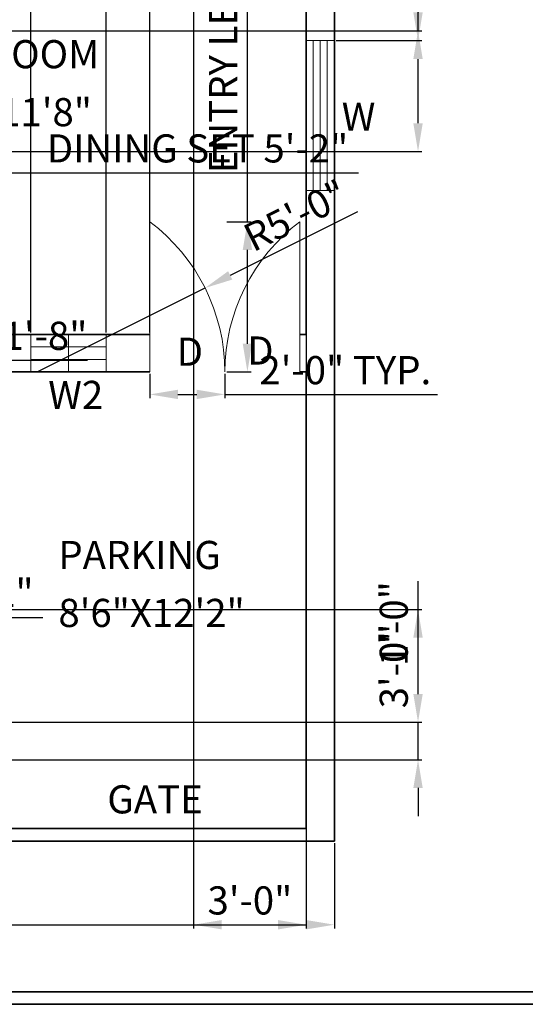
# Model space of a CAD drawing. Units: inches. Extents: x 2436 to 3928, y 1526 to 2149.
# Tile 3 of 6: x 2742 to 2903, y 1526 to 1840. Entities that reach past the tile are written whole.
import ezdxf

# ---------------------------------------------------------------- set-up
doc = ezdxf.new("R2010")
doc.units = ezdxf.units.IN
for name, color, linetype, lineweight in [('A-AREA-IDEN', 152, 'Continuous', 18), ('A-DOOR', 4, 'Continuous', 18), ('A-DOOR-TEXT', 30, 'Continuous', 18), ('A-GLAZ', 2, 'Continuous', 18), ('A-GLAZ-TEXT', 114, 'Continuous', 18), ('A-WALL', 7, 'Continuous', 35), ('G-ANNO-TTLB', 7, 'Continuous', 35), ('S-ANNO-DIMS', 2, 'Continuous', 18)]:
    doc.layers.add(name, color=color, linetype=linetype, lineweight=lineweight)
doc.styles.get("Standard").update_dxf_attribs({"font": 'arial.ttf'})
doc.dimstyles.new('ISO-25', dxfattribs={"dimtxt": 9, "dimasz": 9, "dimexe": 1.25, "dimexo": 0.625, "dimgap": 2, "dimtad": 1, "dimdec": 1, "dimlunit": 4, "dimtxsty": 'Standard', "dimcen": 2.5, "dimadec": 0, "dimazin": 0, "dimtfac": 1, "dimtdec": 1, "dimtmove": 0, "dimatfit": 3, "dimfxl": 1, "dimarcsym": 0})

# ---------------------------------------------------------------- blocks, each defined once
blk = doc.blocks.new('WIN-48x9-PLAN')
for p, q in [((0, 0), (0, 9)), ((0, 6.75), (48, 6.75)), ((48, 0), (48, 9)), ((0, 4.5), (48, 4.5)), ((0, 2.25), (48, 2.25))]:
    blk.add_line(p, q)
blk = doc.blocks.new('DOOR-ENTRY-LEAF-PLAN')
blk.add_line((0, 0), (0, 48))
blk.add_arc((-36, 0), 60, 0, 53.1301)
blk = doc.blocks.new('*D46')
at = {"layer": 'Defpoints', "color": 0, "transparency": 16777216}
for p in [(2807.24, 1775.79), (2814.44, 1775.79), (2807.24, 1727.79)]:
    blk.add_point(p, dxfattribs=at)
at = {"layer": 'S-ANNO-DIMS', "color": 0, "lineweight": -2, "transparency": 16777216}
for p, q in [((2814.44, 1775.79), (2814.44, 1924.22)), ((2807.86, 1775.79), (2815.69, 1775.79)), ((2814.44, 1736.79), (2814.44, 1766.79)), ((2807.86, 1727.79), (2815.69, 1727.79))]:
    blk.add_line(p, q, dxfattribs=at)
at = {"layer": 'S-ANNO-DIMS', "color": 0, "transparency": 16777216}
for points in [[(2812.94, 1766.79), (2815.94, 1766.79), (2814.44, 1775.79)], [(2812.94, 1736.79), (2815.94, 1736.79), (2814.44, 1727.79)]]:
    blk.add_solid(points, dxfattribs=at)
at = {"layer": 'S-ANNO-DIMS', "color": 0, "transparency": 16777216, "insert": (2807.84, 1854.5), "char_height": 9, "attachment_point": 5, "rotation": 90}
blk.add_mtext('ENTRY LEAF 4\'-0" TYP.', dxfattribs=at)
blk = doc.blocks.new('*D47')
at = {"layer": 'Defpoints', "color": 0, "transparency": 16777216}
for p in [(2783.24, 1727.79), (2807.24, 1727.79), (2807.24, 1720.59)]:
    blk.add_point(p, dxfattribs=at)
at = {"layer": 'S-ANNO-DIMS', "color": 0, "lineweight": -2, "transparency": 16777216}
for p, q in [((2783.24, 1727.16), (2783.24, 1719.34)), ((2807.24, 1727.16), (2807.24, 1719.34)), ((2792.24, 1720.59), (2798.24, 1720.59)), ((2807.24, 1720.59), (2875.25, 1720.59))]:
    blk.add_line(p, q, dxfattribs=at)
at = {"layer": 'S-ANNO-DIMS', "color": 0, "transparency": 16777216}
for points in [[(2792.24, 1722.09), (2792.24, 1719.09), (2783.24, 1720.59)], [(2798.24, 1722.09), (2798.24, 1719.09), (2807.24, 1720.59)]]:
    blk.add_solid(points, dxfattribs=at)
at = {"layer": 'S-ANNO-DIMS', "color": 0, "transparency": 16777216, "insert": (2845.74, 1727.18), "char_height": 9, "attachment_point": 5}
blk.add_mtext('2\'-0" TYP.', dxfattribs=at)
blk = doc.blocks.new('*D48')
at = {"layer": 'Defpoints', "color": 0, "transparency": 16777216}
for p in [(2738.03, 1791.43), (2675.93, 1782.12), (2738.03, 1782.12)]:
    blk.add_point(p, dxfattribs=at)
at = {"layer": 'S-ANNO-DIMS', "color": 0, "lineweight": -2, "transparency": 16777216}
for p, q in [((2675.93, 1782.74), (2675.93, 1792.68)), ((2684.93, 1791.43), (2729.03, 1791.43)), ((2738.03, 1782.74), (2738.03, 1792.68)), ((2738.03, 1791.43), (2849.95, 1791.43))]:
    blk.add_line(p, q, dxfattribs=at)
at = {"layer": 'S-ANNO-DIMS', "color": 0, "transparency": 16777216}
for points in [[(2684.93, 1792.93), (2684.93, 1789.93), (2675.93, 1791.43)], [(2729.03, 1792.93), (2729.03, 1789.93), (2738.03, 1791.43)]]:
    blk.add_solid(points, dxfattribs=at)
at = {"layer": 'S-ANNO-DIMS', "color": 0, "transparency": 16777216, "insert": (2798.49, 1798.08), "char_height": 9, "attachment_point": 5}
blk.add_mtext('DINING SET 5\'-2"', dxfattribs=at)
blk = doc.blocks.new('*D50')
at = {"layer": 'Defpoints', "color": 0, "transparency": 16777216}
for p in [(2638.33, 1653.19), (2664.4, 1653.19), (2664.4, 1649.28)]:
    blk.add_point(p, dxfattribs=at)
at = {"layer": 'S-ANNO-DIMS', "color": 0, "lineweight": -2, "transparency": 16777216}
for p, q in [((2638.33, 1652.56), (2638.33, 1648.03)), ((2664.4, 1652.56), (2664.4, 1648.03)), ((2647.33, 1649.28), (2655.4, 1649.28)), ((2664.4, 1649.28), (2749.06, 1649.28))]:
    blk.add_line(p, q, dxfattribs=at)
at = {"layer": 'S-ANNO-DIMS', "color": 0, "transparency": 16777216}
for points in [[(2647.33, 1650.78), (2647.33, 1647.78), (2638.33, 1649.28)], [(2655.4, 1650.78), (2655.4, 1647.78), (2664.4, 1649.28)]]:
    blk.add_solid(points, dxfattribs=at)
at = {"layer": 'S-ANNO-DIMS', "color": 0, "transparency": 16777216, "insert": (2711.23, 1655.93), "char_height": 9, "attachment_point": 5}
blk.add_mtext('RANGE 2\'-2"', dxfattribs=at)
blk = doc.blocks.new('*D55')
at = {"layer": 'Defpoints', "color": 0, "transparency": 16777216}
for p in [(2718.2, 1731.57), (2698.27, 1727.86), (2718.2, 1727.86)]:
    blk.add_point(p, dxfattribs=at)
at = {"layer": 'S-ANNO-DIMS', "color": 0, "lineweight": -2, "transparency": 16777216}
for p, q in [((2689.27, 1731.57), (2680.27, 1731.57)), ((2698.27, 1728.48), (2698.27, 1732.82)), ((2698.27, 1731.57), (2718.2, 1731.57)), ((2718.2, 1728.48), (2718.2, 1732.82)), ((2727.2, 1731.57), (2763.27, 1731.57))]:
    blk.add_line(p, q, dxfattribs=at)
at = {"layer": 'S-ANNO-DIMS', "color": 0, "transparency": 16777216}
for points in [[(2689.27, 1733.07), (2689.27, 1730.07), (2698.27, 1731.57)], [(2727.2, 1733.07), (2727.2, 1730.07), (2718.2, 1731.57)]]:
    blk.add_solid(points, dxfattribs=at)
at = {"layer": 'S-ANNO-DIMS', "color": 0, "transparency": 16777216, "insert": (2749.73, 1738.16), "char_height": 9, "attachment_point": 5}
blk.add_mtext('1\'-8"', dxfattribs=at)
blk = doc.blocks.new('*D56')
at = {"layer": 'Defpoints', "color": 0, "transparency": 16777216}
for p in [(2482.24, 1577.79), (2842.24, 1577.79), (2842.24, 1551.04)]:
    blk.add_point(p, dxfattribs=at)
at = {"layer": 'S-ANNO-DIMS', "color": 0, "lineweight": -2, "transparency": 16777216}
for p, q in [((2482.24, 1577.16), (2482.24, 1549.79)), ((2842.24, 1577.16), (2842.24, 1549.79)), ((2491.24, 1551.04), (2833.24, 1551.04))]:
    blk.add_line(p, q, dxfattribs=at)
at = {"layer": 'S-ANNO-DIMS', "color": 0, "transparency": 16777216}
for points in [[(2491.24, 1552.54), (2491.24, 1549.54), (2482.24, 1551.04)], [(2833.24, 1552.54), (2833.24, 1549.54), (2842.24, 1551.04)]]:
    blk.add_solid(points, dxfattribs=at)
at = {"layer": 'S-ANNO-DIMS', "color": 0, "transparency": 16777216, "insert": (2662.24, 1557.64), "char_height": 9, "attachment_point": 5}
blk.add_mtext('30\'-0"', dxfattribs=at)
blk = doc.blocks.new('*D59')
at = {"layer": 'Defpoints', "color": 0, "transparency": 16777216}
for p in [(2797.24, 2008.79), (2833.24, 2008.79), (2833.24, 1551.04)]:
    blk.add_point(p, dxfattribs=at)
at = {"layer": 'S-ANNO-DIMS', "color": 0, "lineweight": -2, "transparency": 16777216}
for p, q in [((2797.24, 2008.16), (2797.24, 1549.79)), ((2833.24, 2008.16), (2833.24, 1549.79)), ((2806.24, 1551.04), (2824.24, 1551.04))]:
    blk.add_line(p, q, dxfattribs=at)
at = {"layer": 'S-ANNO-DIMS', "color": 0, "transparency": 16777216}
for points in [[(2806.24, 1552.54), (2806.24, 1549.54), (2797.24, 1551.04)], [(2824.24, 1552.54), (2824.24, 1549.54), (2833.24, 1551.04)]]:
    blk.add_solid(points, dxfattribs=at)
at = {"layer": 'S-ANNO-DIMS', "color": 0, "transparency": 16777216, "insert": (2815.24, 1557.64), "char_height": 9, "attachment_point": 5}
blk.add_mtext('3\'-0"', dxfattribs=at)
blk = doc.blocks.new('*D61')
at = {"layer": 'Defpoints', "color": 0, "transparency": 16777216}
for p in [(2842.24, 1922.29), (2842.24, 1833.79), (2868.99, 1833.79)]:
    blk.add_point(p, dxfattribs=at)
at = {"layer": 'S-ANNO-DIMS', "color": 0, "lineweight": -2, "transparency": 16777216}
for p, q in [((2842.86, 1922.29), (2870.24, 1922.29)), ((2868.99, 1913.29), (2868.99, 1842.79)), ((2842.86, 1833.79), (2870.24, 1833.79))]:
    blk.add_line(p, q, dxfattribs=at)
at = {"layer": 'S-ANNO-DIMS', "color": 0, "transparency": 16777216}
for points in [[(2867.49, 1913.29), (2870.49, 1913.29), (2868.99, 1922.29)], [(2867.49, 1842.79), (2870.49, 1842.79), (2868.99, 1833.79)]]:
    blk.add_solid(points, dxfattribs=at)
at = {"layer": 'S-ANNO-DIMS', "color": 0, "transparency": 16777216, "insert": (2862.33, 1878.04), "char_height": 9, "attachment_point": 5, "rotation": 90}
blk.add_mtext('7\'-4 1/2"', dxfattribs=at)
blk = doc.blocks.new('*D63')
at = {"layer": 'Defpoints', "color": 0, "transparency": 16777216}
for p in [(2491.24, 1651.79), (2868.99, 1651.79), (2491.24, 1615.79)]:
    blk.add_point(p, dxfattribs=at)
at = {"layer": 'S-ANNO-DIMS', "color": 0, "lineweight": -2, "transparency": 16777216}
for p, q in [((2491.86, 1651.79), (2870.24, 1651.79)), ((2868.99, 1624.79), (2868.99, 1642.79)), ((2491.86, 1615.79), (2870.24, 1615.79))]:
    blk.add_line(p, q, dxfattribs=at)
at = {"layer": 'S-ANNO-DIMS', "color": 0, "transparency": 16777216}
for points in [[(2867.49, 1642.79), (2870.49, 1642.79), (2868.99, 1651.79)], [(2867.49, 1624.79), (2870.49, 1624.79), (2868.99, 1615.79)]]:
    blk.add_solid(points, dxfattribs=at)
at = {"layer": 'S-ANNO-DIMS', "color": 0, "transparency": 16777216, "insert": (2862.39, 1633.79), "char_height": 9, "attachment_point": 5, "rotation": 90}
blk.add_mtext('3\'-0"', dxfattribs=at)
blk = doc.blocks.new('*D65')
at = {"layer": 'Defpoints', "color": 0, "transparency": 16777216}
for p in [(2575.24, 1615.79), (2868.99, 1615.79), (2575.24, 1603.79)]:
    blk.add_point(p, dxfattribs=at)
at = {"layer": 'S-ANNO-DIMS', "color": 0, "lineweight": -2, "transparency": 16777216}
for p, q in [((2868.99, 1624.79), (2868.99, 1660.87)), ((2575.86, 1615.79), (2870.24, 1615.79)), ((2868.99, 1603.79), (2868.99, 1615.79)), ((2575.86, 1603.79), (2870.24, 1603.79)), ((2868.99, 1594.79), (2868.99, 1585.79))]:
    blk.add_line(p, q, dxfattribs=at)
at = {"layer": 'S-ANNO-DIMS', "color": 0, "transparency": 16777216}
for points in [[(2867.49, 1624.79), (2870.49, 1624.79), (2868.99, 1615.79)], [(2867.49, 1594.79), (2870.49, 1594.79), (2868.99, 1603.79)]]:
    blk.add_solid(points, dxfattribs=at)
at = {"layer": 'S-ANNO-DIMS', "color": 0, "transparency": 16777216, "insert": (2862.39, 1647.33), "char_height": 9, "attachment_point": 5, "rotation": 90}
blk.add_mtext('1\'-0"', dxfattribs=at)
blk = doc.blocks.new('*D68')
at = {"layer": 'Defpoints', "color": 0, "transparency": 16777216}
for p in [(2769.24, 2114.67), (2745.24, 1739.79), (2769.24, 1739.79)]:
    blk.add_point(p, dxfattribs=at)
at = {"layer": 'S-ANNO-DIMS', "color": 0, "lineweight": -2, "transparency": 16777216}
for p, q in [((2745.24, 1740.41), (2745.24, 2115.92)), ((2769.24, 1740.41), (2769.24, 2115.92)), ((2754.24, 2114.67), (2760.24, 2114.67)), ((2769.24, 2114.67), (2806.32, 2114.67))]:
    blk.add_line(p, q, dxfattribs=at)
at = {"layer": 'S-ANNO-DIMS', "color": 0, "transparency": 16777216}
for points in [[(2754.24, 2116.17), (2754.24, 2113.17), (2745.24, 2114.67)], [(2760.24, 2116.17), (2760.24, 2113.17), (2769.24, 2114.67)]]:
    blk.add_solid(points, dxfattribs=at)
at = {"layer": 'S-ANNO-DIMS', "color": 0, "transparency": 16777216, "insert": (2792.28, 2121.26), "char_height": 9, "attachment_point": 5}
blk.add_mtext('2\'-0"', dxfattribs=at)
blk = doc.blocks.new('*D69')
at = {"layer": 'Defpoints', "color": 0, "transparency": 16777216}
for p in [(2783.24, 2114.67), (2769.24, 1739.79), (2783.24, 1739.79)]:
    blk.add_point(p, dxfattribs=at)
at = {"layer": 'S-ANNO-DIMS', "color": 0, "lineweight": -2, "transparency": 16777216}
for p, q in [((2769.24, 1740.41), (2769.24, 2115.92)), ((2783.24, 1740.41), (2783.24, 2115.92)), ((2760.24, 2114.67), (2751.24, 2114.67)), ((2769.24, 2114.67), (2783.24, 2114.67)), ((2792.24, 2114.67), (2828.32, 2114.67))]:
    blk.add_line(p, q, dxfattribs=at)
at = {"layer": 'S-ANNO-DIMS', "color": 0, "transparency": 16777216}
for points in [[(2760.24, 2116.17), (2760.24, 2113.17), (2769.24, 2114.67)], [(2792.24, 2116.17), (2792.24, 2113.17), (2783.24, 2114.67)]]:
    blk.add_solid(points, dxfattribs=at)
at = {"layer": 'S-ANNO-DIMS', "color": 0, "transparency": 16777216, "insert": (2814.78, 2121.19), "char_height": 9, "attachment_point": 5}
blk.add_mtext('1\'-2"', dxfattribs=at)
blk = doc.blocks.new('*D71')
at = {"layer": 'Defpoints', "color": 0, "transparency": 16777216}
for p in [(2577.24, 1836.79), (2868.99, 1836.79), (2577.24, 1798.29)]:
    blk.add_point(p, dxfattribs=at)
at = {"layer": 'S-ANNO-DIMS', "color": 0, "lineweight": -2, "transparency": 16777216}
for p, q in [((2868.99, 1836.79), (2868.99, 1894.68)), ((2577.86, 1836.79), (2870.24, 1836.79)), ((2868.99, 1807.29), (2868.99, 1827.79)), ((2577.86, 1798.29), (2870.24, 1798.29))]:
    blk.add_line(p, q, dxfattribs=at)
at = {"layer": 'S-ANNO-DIMS', "color": 0, "transparency": 16777216}
for points in [[(2867.49, 1827.79), (2870.49, 1827.79), (2868.99, 1836.79)], [(2867.49, 1807.29), (2870.49, 1807.29), (2868.99, 1798.29)]]:
    blk.add_solid(points, dxfattribs=at)
at = {"layer": 'S-ANNO-DIMS', "color": 0, "transparency": 16777216, "insert": (2862.33, 1870.23), "char_height": 9, "attachment_point": 5, "rotation": 90}
blk.add_mtext('3\'-2 1/2"', dxfattribs=at)
blk = doc.blocks.new('*D81')
at = {"layer": 'Defpoints', "color": 0, "transparency": 16777216}
for p in [(2800.9, 1754.62), (2747.24, 1727.79)]:
    blk.add_point(p, dxfattribs=at)
at = {"layer": 'S-ANNO-DIMS', "color": 0, "lineweight": -2, "transparency": 16777216}
for p, q in [((2849.68, 1779.01), (2808.95, 1758.65)), ((2747.24, 1727.79), (2800.9, 1754.62))]:
    blk.add_line(p, q, dxfattribs=at)
at = {"layer": 'S-ANNO-DIMS', "color": 0, "transparency": 16777216}
blk.add_solid([(2808.28, 1759.99), (2809.62, 1757.31), (2800.9, 1754.62)], dxfattribs=at)
at = {"layer": 'S-ANNO-DIMS', "color": 0, "transparency": 16777216, "insert": (2830.39, 1776.74), "char_height": 9, "attachment_point": 5, "rotation": 26.5648}
blk.add_mtext('R5\'-0"', dxfattribs=at)

msp = doc.modelspace()

# ---------------------------------------------------------------- linework, layer by layer
at = {"layer": 'A-GLAZ'}
for p, q in [((2745.24, 1727.79), (2745.24, 1739.79)), ((2757.24, 1727.79), (2757.24, 1739.79)), ((2769.24, 1727.79), (2769.24, 1739.79)), ((2745.24, 1735.79), (2769.24, 1735.79)), ((2745.24, 1731.79), (2769.24, 1731.79))]:
    msp.add_line(p, q, dxfattribs=at)
at = {"layer": 'A-WALL'}
for p, q in [((2842.24, 2017.79), (2842.24, 1585.79)), ((2833.24, 1739.79), (2833.24, 1879.79)), ((2842.24, 1744.79), (2842.24, 1732.79)), ((2647.24, 1739.79), (2783.24, 1739.79)), ((2831.24, 1739.79), (2833.24, 1739.79)), ((2842.24, 1732.79), (2842.24, 1577.79)), ((2731.24, 1727.79), (2783.24, 1727.79)), ((2831.24, 1727.79), (2833.24, 1727.79)), ((2833.24, 1581.79), (2833.24, 1727.79)), ((2491.24, 1581.79), (2833.24, 1581.79)), ((2482.24, 1577.79), (2842.24, 1577.79))]:
    msp.add_line(p, q, dxfattribs=at)
at = {"layer": 'G-ANNO-TTLB'}
for points in [[(2436, 2138.4), (3927.51, 2138.4), (3927.51, 1525.6), (2436, 1525.6)], [(2440, 2134.4), (3923.51, 2134.4), (3923.51, 1529.6), (2440, 1529.6)]]:
    msp.add_lwpolyline(points, close=True, dxfattribs=at)

# ---------------------------------------------------------------- block references
at = {"layer": 'A-DOOR'}
msp.add_blockref('DOOR-ENTRY-LEAF-PLAN', (2783.24, 1727.79), dxfattribs=at)
at = {"layer": 'A-DOOR', "extrusion": (0, 0, -1), "zscale": -1}
msp.add_blockref('DOOR-ENTRY-LEAF-PLAN', (-2831.24, 1727.79), dxfattribs=at)
at = {"layer": 'A-GLAZ', "rotation": 270.0000000000039}
msp.add_blockref('WIN-48x9-PLAN', (2833.24, 1833.79), dxfattribs=at)

# ---------------------------------------------------------------- texts
at = {"layer": 'A-AREA-IDEN'}
for s, p in [('LIVING ROOM', (2690.1, 1824.87)), ('   18\'2"X11\'8"', (2690.1, 1806.33)), ('PARKING', (2754.01, 1664.76)), ('8\'6"X12\'2"', (2754.01, 1646.23))]:
    msp.add_text(s, height=9, dxfattribs=at).set_placement(p)
at = {"layer": 'A-DOOR-TEXT'}
for s, p in [('D', (2791.82, 1729.75)), ('D', (2814.36, 1730.12)), ('GATE', (2769.64, 1586.63))]:
    msp.add_text(s, height=9, dxfattribs=at).set_placement(p)
at = {"layer": 'A-GLAZ-TEXT'}
for s, p in [('W', (2844.59, 1804.92)), ('W2', (2750.74, 1715.93))]:
    msp.add_text(s, height=9, dxfattribs=at).set_placement(p)

# ---------------------------------------------------------------- dimensions: what is measured, and where the dimension line sits
at = {"layer": 'S-ANNO-DIMS'}
for base, p1, p2, picture, middle in [((2769.24, 2114.67), (2745.24, 1739.79), (2769.24, 1739.79), '*D68', (2792.28, 2121.26)), ((2783.24, 2114.67), (2769.24, 1739.79), (2783.24, 1739.79), '*D69', (2814.78, 2121.19)), ((2833.24, 1551.04), (2797.24, 2008.79), (2833.24, 2008.79), '*D59', (2815.24, 1557.64)), ((2718.2, 1731.57), (2698.27, 1727.86), (2718.2, 1727.86), '*D55', (2749.73, 1738.16)), ((2842.24, 1551.04), (2482.24, 1577.79), (2842.24, 1577.79), '*D56', (2662.24, 1557.64))]:
    dim = msp.add_linear_dim(base=base, p1=p1, p2=p2, dimstyle='ISO-25', override={"dimdec": 1, "dimlfac": 1, "dimrnd": 0, "dimzin": 1, "dimdsep": 46, "dimlunit": 4, "dimfrac": 2}, dxfattribs=at)
    dim.commit()
    dim.dimension.update_dxf_attribs({"geometry": picture, "text_midpoint": middle})
dim = msp.add_linear_dim(base=(2814.44, 1775.79), p1=(2807.24, 1727.79), p2=(2807.24, 1775.79), angle=90, text='ENTRY LEAF <> TYP.', dimstyle='ISO-25', override={"dimdec": 1, "dimlfac": 1, "dimrnd": 0, "dimzin": 1, "dimdsep": 46, "dimlunit": 4, "dimfrac": 2}, dxfattribs=at)
dim.commit()
dim.dimension.update_dxf_attribs({"geometry": '*D46', "text_midpoint": (2807.84, 1854.5)})
for base, p1, p2, picture, middle in [((2868.99, 1833.79), (2842.24, 1922.29), (2842.24, 1833.79), '*D61', (2862.33, 1878.04)), ((2868.99, 1836.79), (2577.24, 1798.29), (2577.24, 1836.79), '*D71', (2862.33, 1870.23)), ((2868.99, 1615.79), (2575.24, 1603.79), (2575.24, 1615.79), '*D65', (2862.39, 1647.33)), ((2868.99, 1651.79), (2491.24, 1615.79), (2491.24, 1651.79), '*D63', (2862.39, 1633.79))]:
    dim = msp.add_linear_dim(base=base, p1=p1, p2=p2, angle=90, dimstyle='ISO-25', override={"dimdec": 1, "dimlfac": 1, "dimrnd": 0, "dimzin": 1, "dimdsep": 46, "dimlunit": 4, "dimfrac": 2}, dxfattribs=at)
    dim.commit()
    dim.dimension.update_dxf_attribs({"geometry": picture, "text_midpoint": middle})
for base, p1, p2, text, picture, middle in [((2738.03, 1791.43), (2675.93, 1782.12), (2738.03, 1782.12), 'DINING SET <>', '*D48', (2798.49, 1798.08)), ((2807.24, 1720.59), (2783.24, 1727.79), (2807.24, 1727.79), '<> TYP.', '*D47', (2845.74, 1727.18)), ((2664.4, 1649.28), (2638.33, 1653.19), (2664.4, 1653.19), 'RANGE <>', '*D50', (2711.23, 1655.93))]:
    dim = msp.add_linear_dim(base=base, p1=p1, p2=p2, text=text, dimstyle='ISO-25', override={"dimdec": 1, "dimlfac": 1, "dimrnd": 0, "dimzin": 1, "dimdsep": 46, "dimlunit": 4, "dimfrac": 2}, dxfattribs=at)
    dim.commit()
    dim.dimension.update_dxf_attribs({"geometry": picture, "text_midpoint": middle})
dim = msp.add_radius_dim(center=(2747.24, 1727.79), mpoint=(2800.9, 1754.62), dimstyle='ISO-25', override={"dimdec": 1, "dimlfac": 1, "dimrnd": 0, "dimzin": 1, "dimdsep": 46, "dimlunit": 4, "dimfrac": 2}, dxfattribs=at)
dim.commit()
dim.dimension.update_dxf_attribs({"geometry": '*D81', "text_midpoint": (2830.39, 1776.74)})

doc.saveas('drawing.dxf')
